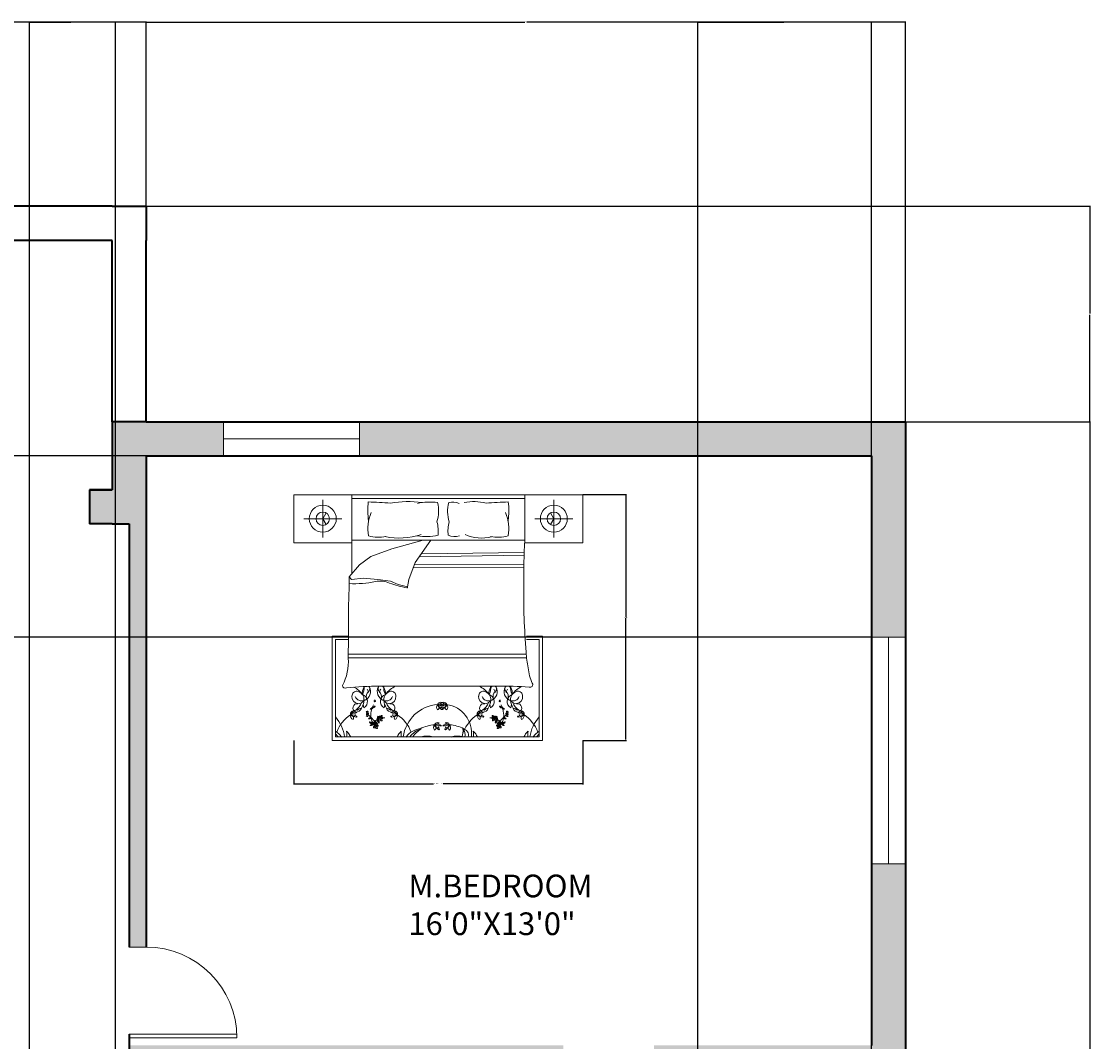
# Model space of a CAD drawing. Units: inches. Extents: x -26 to 13070, y -956 to 6917.
# Tile 11 of 13: x 314 to 597, y -154 to 116. Entities that reach past the tile are written whole.
import ezdxf

# ---------------------------------------------------------------- set-up
doc = ezdxf.new("R2010")
doc.units = ezdxf.units.IN
doc.header["$MEASUREMENT"] = 0
for name, color, linetype, lineweight in [('A-ANNO-DIMS', 2, 'Continuous', 18), ('A-AREA-IDEN', 7, 'Continuous', 18), ('A-DOOR', 3, 'Continuous', 18), ('A-FURN', 8, 'Continuous', 13), ('A-GLAZ', 4, 'Continuous', 18), ('A-WALL', 7, 'Continuous', 35), ('A-WALL-PATT', 252, 'Continuous', 13)]:
    doc.layers.add(name, color=color, linetype=linetype, lineweight=lineweight)
doc.styles.get("Standard").update_dxf_attribs({"font": 'arial.ttf'})
doc.dimstyles.get("Standard").update_dxf_attribs({"dimtxt": 0.18, "dimasz": 0.18, "dimexe": 0.18, "dimexo": 0.0625, "dimgap": 0.09, "dimtad": 0, "dimtih": 1, "dimtoh": 1, "dimdec": 0, "dimzin": 0, "dimdsep": 46, "dimlunit": 3, "dimtxsty": 'Standard', "dimcen": 0.09, "dimadec": 0, "dimazin": 0, "dimtfac": 1, "dimtdec": 0, "dimtofl": 0, "dimtmove": 0, "dimatfit": 3, "dimfxl": 1, "dimtolj": 1, "dimtzin": 0, "dimarcsym": 0})

# ---------------------------------------------------------------- blocks, each defined once
blk = doc.blocks.new('BED-DOUBLE-NIGHTSTANDS')
for p, q in [((0, 65), (76.43, 65)), ((7.64, 53.64), (7.64, 63.62)), ((15.29, 65), (15.29, 44.02)), ((61.14, 64.02), (15.29, 64.02)), ((68.79, 53.64), (68.79, 63.62)), ((12.64, 58.63), (2.65, 58.63)), ((63.79, 58.63), (73.78, 58.63)), ((15.29, 52.92), (61.14, 52.92)), ((25.9, 50.65), (34.24, 52.92)), ((36.28, 52.92), (32.09, 47.09)), ((17.39, 46.47), (20.33, 48.64)), ((20.33, 48.64), (25.9, 50.65)), ((60.91, 48.96), (33.16, 48.57)), ((60.94, 49.74), (33.73, 49.36)), ((14.6, 43.22), (17.39, 46.47)), ((32.09, 47.09), (30.39, 42.6)), ((60.87, 45.77), (31.55, 45.65)), ((60.87, 46.55), (31.85, 46.44)), ((15.22, 42.6), (14.6, 43.22)), ((18.32, 42.91), (15.22, 42.6)), ((22.19, 42.6), (18.32, 42.91)), ((25.59, 42.14), (22.19, 42.6)), ((30.39, 42.6), (30.08, 40.59)), ((27.6, 41.21), (25.59, 42.14)), ((30.08, 40.59), (27.6, 41.21)), ((10.09, 27.53), (14.41, 27.53)), ((10.09, 0), (10.09, 27.53)), ((14.41, 26.65), (10.97, 26.65)), ((10.97, 26.65), (10.97, 0.89)), ((64.92, 26.65), (61.55, 26.65)), ((61.57, 27.53), (65.81, 27.53)), ((64.92, 0.89), (64.92, 26.65)), ((65.81, 27.53), (65.81, 0)), ((61.49, 22.77), (14.41, 22.77)), ((61.56, 21.81), (14.4, 21.81)), ((53.73, 14.3), (22.7, 14.3)), ((18.51, 8.63), (18.34, 9.5)), ((23.85, 8.63), (24.02, 9.5)), ((52.05, 8.63), (51.88, 9.5)), ((57.39, 8.63), (57.56, 9.5)), ((10.97, 0.89), (64.92, 0.89)), ((65.81, 0), (10.09, 0))]:
    blk.add_line(p, q)
for points in [[(15.29, 52.26), (0, 52.26), (0, 65)], [(61.14, 65), (61.14, 52.26), (76.43, 52.26), (76.43, 65)], [(7.64, 58.63), (8.53, 60.17)], [(68.79, 58.63), (67.89, 60.17)], [(7.64, 58.63), (8.53, 57.08)], [(68.79, 58.63), (67.89, 57.08)]]:
    blk.add_lwpolyline(points)
for points in [[(19.68, 63.09, 0.074897), (19.77, 58.1, -0.472817)], [(37.86, 57.82, 0.14099), (38.01, 62.91, 0.235245)], [(41.12, 57.82, -0.14099), (40.97, 62.91, -0.235245)], [(56.75, 63.09, -0.074897), (56.66, 58.1, 0.472817)], [(14.44, 36.22, 0.001242), (14.4, 21.72, -0.127202), (12.87, 14.5)], [(61.47, 23.37, 0.056112), (62.02, 19.16, 0.095341), (63.1, 15.11)]]:
    blk.add_lwpolyline(points, format="xyb")
for centre, radius in [((7.64, 58.63), 3.57), ((7.64, 58.63), 1.78), ((68.79, 58.63), 3.57), ((68.79, 58.63), 1.78), ((22.92, 5.86), 0.195), ((52.98, 5.86), 0.195), ((21.65, 3.81), 0.195), ((54.25, 3.81), 0.195)]:
    blk.add_circle(centre, radius)
for centre, radius, start, end in [((61.8, 790.45), 728.57, 266.68521, 267.14978), ((30.15, 35.44), 27.72, 82.2196, 99.497), ((36, 49.44), 13.62, 81.5249, 103.96), ((42.02, 59.28), 3.78, 63.3437, 106.1026), ((47.68, 49.72), 13.44, 76.3427, 101.1841), ((14.63, 790.45), 728.57, 272.85022, 273.31479), ((29.41, 56.1), 9.85, 155.1316, 191.7583), ((47.02, 56.1), 9.85, 348.2417, 24.8684), ((28.85, 55.27), 9.36, 354.0129, 15.8293), ((50.13, 55.27), 9.36, 164.1707, 185.9871), ((22.4, 63.99), 10.24, 255.1039, 281.0369), ((27.79, 71.27), 17.76, 258.0397, 289.2615), ((34.99, 67.39), 13.48, 259.8617, 283.6238), ((42.53, 57.96), 4.05, 245.0183, 288.5407), ((49.61, 63.23), 9.73, 243.8761, 286.1746), ((54.03, 63.99), 10.24, 258.9631, 284.8961), ((198.16, 43.58), 137.33, 176.1, 180.9282), ((-55.48, 41.32), 70.1, 355.8294, 1.553), ((15.91, 70.29), 28.85, 267.4519, 281.3392), ((22.8, 35.91), 6.22, 66.2616, 101.3392), ((35.39, 69.47), 29.64, 250.1194, 259.3383), ((29.91, 40.53), 0.184, 268.8623, 19.7536), ((239.96, 38.59), 179.14, 179.1145, 184.8735), ((13.58, 14.54), 0.705, 183.98, 297.3412), ((21.79, -65.25), 79.56, 89.3433, 95.6887), ((15.4, 13.74), 3.17, 328.8218, 9.1554), ((19.32, 13.46), 0.92, 120.0293, 142.325), ((19.32, 13.46), 0.92, 44.4517, 63.558), ((23.03, 13.46), 0.92, 113.229, 135.5483), ((23.03, 13.46), 0.92, 37.675, 66.7144), ((26.95, 13.74), 3.17, 169.7133, 211.1782), ((29.07, 8.92), 5.78, 111.4941, 146.3329), ((46.82, 8.92), 5.78, 33.6671, 68.5059), ((48.94, 13.74), 3.17, 328.8218, 10.2867), ((52.87, 13.46), 0.92, 113.2856, 142.325), ((52.87, 13.46), 0.92, 44.4517, 66.7144), ((56.07, -60.03), 74.37, 85.2402, 91.8035), ((56.57, 13.46), 0.92, 106.6343, 135.5483), ((56.57, 13.46), 0.92, 37.675, 72.5814), ((60.5, 13.74), 3.17, 169.249, 211.1782), ((62.62, 8.92), 5.78, 113.6453, 146.3329), ((62.52, 14.72), 0.697, 246.5219, 33.8264), ((17.18, 11.52), 1.83, 174.9449, 262.8857), ((16.65, 11.7), 1.29, 84.4856, 181.0538), ((13.28, 8.92), 5.78, 33.6671, 63.2997), ((17.9, 12.21), 1.77, 201.5819, 291.4221), ((16.25, 10.75), 2.3, 355.2933, 76.921), ((21.03, 12.36), 2.95, 145.785, 184.7304), ((17.56, 10.28), 1.9, 299.9085, 73.1337), ((17.85, 12.92), 2.44, 289.2822, 29.1751), ((20.73, 11.61), 1.57, 131.5653, 195.1471), ((17.48, 12.48), 2.2, 7.436, 29.9149), ((18.93, 13.64), 1.14, 311.5653, 23.8354), ((24.5, 12.92), 2.44, 150.8249, 250.7178), ((23.42, 13.64), 1.14, 156.1646, 228.4347), ((21.62, 11.61), 1.57, 344.8529, 48.4347), ((24.87, 12.48), 2.2, 150.0851, 172.564), ((24.79, 10.28), 1.9, 106.8663, 240.0915), ((21.32, 12.36), 2.95, 355.2696, 34.215), ((26.1, 10.75), 2.3, 103.079, 184.7067), ((24.46, 12.21), 1.77, 248.5779, 338.4181), ((25.17, 11.52), 1.83, 277.1143, 5.0551), ((25.7, 11.7), 1.29, 358.9462, 95.5144), ((50.72, 11.52), 1.83, 174.9449, 262.8857), ((50.19, 11.7), 1.29, 84.4856, 181.0538), ((51.44, 12.21), 1.77, 201.5819, 291.4221), ((49.8, 10.75), 2.3, 355.2933, 76.921), ((54.57, 12.36), 2.95, 145.785, 184.7304), ((51.1, 10.28), 1.9, 299.9085, 73.1337), ((51.4, 12.92), 2.44, 289.2822, 29.1751), ((54.28, 11.61), 1.57, 131.5653, 195.1471), ((51.03, 12.48), 2.2, 7.436, 29.9149), ((52.48, 13.64), 1.14, 311.5653, 23.8354), ((58.04, 12.92), 2.44, 150.8249, 250.7178), ((56.96, 13.64), 1.14, 156.1646, 228.4347), ((55.16, 11.61), 1.57, 344.8529, 48.4347), ((58.41, 12.48), 2.2, 150.0851, 172.564), ((58.34, 10.28), 1.9, 106.8663, 240.0915), ((54.87, 12.36), 2.95, 355.2696, 34.215), ((59.64, 10.75), 2.3, 103.079, 184.7067), ((58, 12.21), 1.77, 248.5779, 338.4181), ((58.72, 11.52), 1.83, 277.1143, 5.0551), ((59.25, 11.7), 1.29, 358.9462, 95.5144), ((16.76, 8.57), 1.15, 80.264, 250.8688), ((14.48, 11.1), 3.61, 301.2614, 341.7045), ((16.48, 8.92), 1.43, 265.969, 344.3045), ((18.02, 7.01), 1.53, 96.1662, 141.5825), ((16.86, 11.92), 2.22, 272.3591, 324.0401), ((14.45, 10.81), 4.1, 326.2883, 356.5076), ((21.03, 12.36), 2.95, 212.7011, 216.3445), ((18.76, 11.08), 0.474, 257.3041, 15.1471), ((19.71, 9.44), 1.23, 308.2101, 316.3071), ((20.47, 8.64), 0.367, 278.3432, 4.2869), ((20.26, 8.96), 0.641, 300.656, 332.6341), ((20.74, 8.53), 0.156, 55.7657, 157.4417), ((26.69, 6.51), 6.33, 153.0032, 159.8941), ((20.99, 8.68), 0.156, 84.3784, 186.0543), ((20.84, 9.3), 0.641, 269.1859, 301.164), ((21.03, 8.97), 0.367, 237.5332, 323.4768), ((20.67, 10.02), 1.23, 285.5129, 293.6099), ((20.55, 9.79), 1.21, 301.164, 321.5612), ((21.48, 8.64), 0.401, 87.3579, 140.4944), ((21.4, 10.36), 0.147, 102.7051, 280.4384), ((19.56, 10), 2.16, 324.6898, 333.4936), ((21.38, 10.45), 0.24, 280.4384, 100.4136), ((23.59, 11.08), 0.474, 164.8529, 282.6959), ((21.32, 12.36), 2.95, 323.6555, 327.2989), ((25.49, 11.92), 2.22, 215.9599, 267.6409), ((27.9, 10.81), 4.1, 183.4924, 213.7117), ((27.87, 11.1), 3.61, 198.2955, 238.7386), ((24.33, 7.01), 1.53, 38.4175, 83.8338), ((25.87, 8.92), 1.43, 195.6955, 274.031), ((25.59, 8.57), 1.15, 289.1312, 99.736), ((38.81, -0.46), 9.98, 94.4623, 172.255), ((38.85, 8.75), 1.11, 137.7873, 219.1145), ((37.6, 8.78), 0.834, 298.5391, 58.3627), ((38.83, 9.26), 0.827, 63.0274, 163.8037), ((37.99, 11.2), 1.7, 271.4585, 315.3727), ((38.68, 8.05), 1.58, 45.5411, 114.3101), ((40.12, 16.15), 6.98, 252.593, 267.2582), ((38.85, 9.46), 0.816, 177.7585, 283.852), ((40.42, 10.31), 2.52, 198.9159, 238.011), ((39.76, 8.05), 1.58, 65.6899, 134.4589), ((38.32, 16.15), 6.98, 272.7418, 287.407), ((39.02, 8.77), 0.108, 283.852, 219.9245), ((39.62, 9.26), 0.827, 16.1963, 116.9726), ((40.45, 11.2), 1.7, 224.6273, 268.5415), ((39.42, 8.81), 0.0651, 320.1909, 256.0209), ((38.02, 10.31), 2.52, 301.989, 341.0841), ((39.6, 9.46), 0.816, 256.148, 2.2415), ((40.85, 8.78), 0.834, 121.6373, 241.4609), ((39.59, 8.75), 1.11, 320.8855, 42.2127), ((39.31, 1.85), 7.72, 352.8636, 81.8197), ((50.3, 8.57), 1.15, 80.264, 250.8688), ((48.03, 11.1), 3.61, 301.2614, 341.7045), ((50.03, 8.92), 1.43, 265.969, 344.3045), ((51.57, 7.01), 1.53, 96.1662, 141.5825), ((50.4, 11.92), 2.22, 272.3591, 324.0401), ((47.99, 10.81), 4.1, 326.2883, 356.5076), ((54.57, 12.36), 2.95, 212.7011, 216.3445), ((52.3, 11.08), 0.474, 257.3041, 15.1471), ((54.52, 10.45), 0.24, 79.5864, 259.5616), ((55.35, 9.79), 1.21, 218.4388, 238.836), ((54.42, 8.64), 0.401, 39.5056, 92.6421), ((56.33, 10), 2.16, 206.5064, 215.3102), ((54.5, 10.36), 0.147, 259.5616, 77.2949), ((54.87, 8.97), 0.367, 216.5232, 302.4668), ((55.05, 9.3), 0.641, 238.836, 270.8141), ((55.22, 10.02), 1.23, 246.3901, 254.4871), ((49.2, 6.51), 6.33, 20.1059, 26.9968), ((54.91, 8.68), 0.156, 353.9457, 95.6216), ((55.15, 8.53), 0.156, 22.5583, 124.2343), ((55.43, 8.64), 0.367, 175.7131, 261.6568), ((55.63, 8.96), 0.641, 207.3659, 239.344), ((56.18, 9.44), 1.23, 223.6929, 231.7899), ((57.13, 11.08), 0.474, 164.8529, 282.6959), ((54.87, 12.36), 2.95, 323.6555, 327.2989), ((59.04, 11.92), 2.22, 215.9599, 267.6409), ((61.45, 10.81), 4.1, 183.4924, 213.7117), ((61.41, 11.1), 3.61, 198.2955, 238.7386), ((59.41, 8.92), 1.43, 195.6955, 274.031), ((57.87, 7.01), 1.53, 38.4175, 83.8338), ((59.14, 8.57), 1.15, 289.1312, 99.736), ((3.54, -0.46), 9.98, 7.745, 41.8856), ((20.62, -1.45), 9.98, 124.3865, 158.5908), ((15.79, 6.99), 0.827, 92.9516, 193.728), ((16.06, 6.55), 1.11, 167.7115, 249.0387), ((14.09, 8.25), 1.7, 301.3827, 345.2969), ((16.26, 5.87), 1.58, 75.4653, 144.2343), ((13.47, 13.61), 6.98, 282.5173, 297.1824), ((14.96, 5.96), 0.834, 328.4633, 88.2869), ((16.64, 8.69), 2.52, 228.8402, 267.9352), ((15.7, 7.17), 0.816, 207.6827, 313.7762), ((16.52, 7.33), 0.703, 63.9755, 143.2681), ((16.19, 6.66), 0.108, 313.7762, 249.7183), ((16.54, 6.35), 0.0602, 101.4834, 217.9409), ((16.56, 6.29), 0.124, 267.9352, 101.4834), ((19.42, 7.32), 0.325, 101.5637, 142.6358), ((19.15, 7.02), 0.195, 273.2768, 86.7232), ((19.41, 6.66), 0.321, 217.7621, 259.0403), ((19.37, 7.21), 0.186, 91.1081, 181.8675), ((19.76, 7.09), 0.591, 203.4276, 227.6104), ((19.57, 6.83), 0.402, 80.3487, 133.6538), ((19.5, 7.16), 0.318, 229.7889, 317.6792), ((19.16, 7.58), 0.468, 288.7263, 352.5032), ((19.14, 6.49), 0.452, 355.053, 68.3618), ((19.5, 6.41), 0.637, 83.0852, 105.7171), ((19.47, 7.55), 0.15, 345.2356, 144.9248), ((19.44, 6.46), 0.149, 232.4737, 355.053), ((15.08, 1.13), 7.26, 43.1541, 52.0459), ((19.61, 7.06), 0.168, 317.6792, 80.3487), ((20.1, 5.51), 0.401, 101.3256, 154.4621), ((19.52, 6.87), 1.21, 280.2588, 300.656), ((19.8, 7.84), 2.16, 268.3264, 277.1302), ((19.26, 6.87), 1.23, 308.2101, 316.3071), ((20.01, 6.06), 0.367, 278.3432, 4.2869), ((19.81, 6.39), 0.641, 300.656, 332.6341), ((20.29, 5.96), 0.156, 55.7657, 157.4417), ((20.55, 8.08), 0.401, 101.3256, 154.4621), ((19.97, 9.45), 1.21, 280.2588, 300.656), ((20.25, 10.41), 2.16, 268.3264, 277.1302), ((26.69, 6.51), 6.33, 163.5842, 183.8277), ((23.54, 6.35), 3.17, 184.756, 209.2041), ((28.11, 13.11), 10.44, 222.2412, 232.1744), ((21.43, 6.15), 0.887, 304.5369, 16.3699), ((21.9, 5.96), 0.539, 272.8499, 356.1226), ((21.52, 5.75), 0.522, 321.7607, 7.9252), ((22.66, 5.9), 0.628, 127.3105, 187.9252), ((21.8, 5.98), 0.645, 355.0106, 41.658), ((22.87, 5.28), 0.614, 104.7558, 148.0499), ((22.71, 6.14), 0.265, 126.1046, 271.4281), ((22.68, 6.21), 0.191, 353.7526, 131.7054), ((22.63, 5.7), 0.129, 262.906, 7.132), ((22.5, 5.98), 0.268, 0.0645, 61.1507), ((22.56, 6.21), 0.306, 311.8413, 355.7877), ((23.19, 6.17), 0.325, 101.5637, 176.365), ((23.15, 6.05), 0.186, 91.1081, 181.8675), ((23.53, 5.93), 0.591, 203.4276, 227.6104), ((23.35, 5.67), 0.402, 80.3487, 133.6538), ((23.27, 6.01), 0.318, 229.7889, 317.6792), ((22.93, 6.42), 0.468, 288.7263, 352.5032), ((22.91, 5.33), 0.452, 355.053, 68.3618), ((23.27, 5.26), 0.637, 83.0852, 105.7171), ((23.25, 6.4), 0.15, 345.2356, 144.9248), ((23.38, 5.91), 0.168, 317.6792, 80.3487), ((23.87, 2.14), 3.81, 87.1071, 94.7585), ((25.83, 7.33), 0.703, 36.7319, 116.0245), ((25.8, 6.29), 0.124, 78.5166, 272.0648), ((26.09, 5.87), 1.58, 35.7657, 104.5347), ((28.88, 13.61), 6.98, 242.8176, 257.4827), ((25.71, 8.69), 2.52, 272.0648, 311.1598), ((25.81, 6.35), 0.0602, 322.0591, 78.5166), ((26.65, 7.17), 0.816, 226.2238, 332.3173), ((26.17, 6.7), 0.0651, 290.2667, 226.2271), ((27.4, 5.96), 0.834, 91.7131, 211.5367), ((26.57, 6.99), 0.827, 346.272, 87.0484), ((28.26, 8.25), 1.7, 194.7031, 238.6173), ((26.29, 6.55), 1.11, 290.9613, 12.2885), ((21.73, -1.45), 9.98, 21.4092, 55.6135), ((39.15, 8.27), 0.124, 238.011, 71.5592), ((39.17, 8.33), 0.0602, 71.5592, 188.0167), ((39.29, 8.27), 0.124, 108.4408, 301.989), ((39.27, 8.33), 0.0602, 351.9833, 108.4408), ((54.16, -1.45), 9.98, 124.3865, 158.5908), ((49.33, 6.99), 0.827, 92.9516, 193.728), ((49.61, 6.55), 1.11, 167.7115, 249.0387), ((47.64, 8.25), 1.7, 301.3827, 345.2969), ((49.81, 5.87), 1.58, 75.4653, 144.2343), ((47.01, 13.61), 6.98, 282.5173, 297.1824), ((49.25, 7.17), 0.816, 207.6827, 313.7762), ((50.19, 8.69), 2.52, 228.8402, 267.9352), ((48.5, 5.96), 0.834, 328.4633, 88.2869), ((50.06, 7.33), 0.703, 63.9755, 143.2681), ((49.74, 6.66), 0.108, 313.7762, 249.7183), ((50.09, 6.35), 0.0602, 101.4834, 217.9409), ((50.1, 6.29), 0.124, 267.9352, 101.4834), ((52.03, 2.14), 3.81, 85.2415, 92.8929), ((52.51, 5.91), 0.168, 99.6513, 222.3208), ((52.62, 6.01), 0.318, 222.3208, 310.2111), ((52.55, 5.67), 0.402, 46.3462, 99.6513), ((52.65, 6.4), 0.15, 35.0752, 194.7644), ((52.97, 6.42), 0.468, 187.4968, 251.2737), ((52.98, 5.33), 0.452, 111.6382, 184.947), ((52.63, 5.26), 0.637, 74.2829, 96.9148), ((52.75, 6.05), 0.186, 358.1325, 88.8919), ((52.36, 5.93), 0.591, 312.3896, 336.5724), ((52.71, 6.17), 0.325, 3.635, 78.4363), ((53.22, 6.21), 0.191, 48.2946, 186.2474), ((53.34, 6.21), 0.306, 184.2123, 228.1587), ((53.4, 5.98), 0.268, 118.8493, 179.9355), ((53.26, 5.7), 0.129, 172.868, 277.094), ((53.19, 6.14), 0.265, 268.5719, 53.8954), ((53.03, 5.28), 0.614, 31.9501, 75.2442), ((54.1, 5.98), 0.645, 138.342, 184.9894), ((53.99, 5.96), 0.539, 183.8774, 267.1501), ((54.47, 6.15), 0.887, 163.6301, 235.4631), ((53.23, 5.9), 0.628, 352.0748, 52.6895), ((54.37, 5.75), 0.522, 172.0748, 218.2393), ((47.79, 13.11), 10.44, 307.8256, 317.7588), ((52.36, 6.35), 3.17, 330.7959, 355.244), ((49.2, 6.51), 6.33, 356.1723, 16.4158), ((55.92, 9.45), 1.21, 239.344, 259.7412), ((55.64, 10.41), 2.16, 262.8698, 271.6736), ((55.34, 8.08), 0.401, 25.5379, 78.6744), ((60.81, 1.13), 7.26, 127.9541, 136.8459), ((55.61, 5.96), 0.156, 22.5583, 124.2343), ((55.88, 6.06), 0.367, 175.7131, 261.6568), ((56.09, 6.39), 0.641, 207.3659, 239.344), ((56.64, 6.87), 1.23, 223.6929, 231.7899), ((56.38, 6.87), 1.21, 239.344, 259.7412), ((56.1, 7.84), 2.16, 262.8698, 271.6736), ((55.8, 5.51), 0.401, 25.5379, 78.6744), ((56.28, 7.06), 0.168, 99.6513, 222.3208), ((56.4, 7.16), 0.318, 222.3208, 310.2111), ((56.32, 6.83), 0.402, 46.3462, 99.6513), ((56.42, 7.55), 0.15, 35.0752, 194.7644), ((56.74, 7.58), 0.468, 187.4968, 251.2737), ((56.76, 6.49), 0.452, 111.6382, 184.947), ((56.45, 6.46), 0.149, 184.947, 307.5263), ((56.4, 6.41), 0.637, 74.2829, 96.9148), ((56.52, 7.21), 0.186, 358.1325, 88.8919), ((56.14, 7.09), 0.591, 312.3896, 336.5724), ((56.48, 7.32), 0.325, 37.3642, 78.4363), ((56.48, 6.66), 0.321, 280.9597, 322.2379), ((56.75, 7.02), 0.195, 93.2768, 266.7232), ((59.37, 7.33), 0.703, 36.7319, 116.0245), ((59.34, 6.29), 0.124, 78.5166, 272.0648), ((59.63, 5.87), 1.58, 35.7657, 104.5347), ((62.43, 13.61), 6.98, 242.8176, 257.4827), ((59.25, 8.69), 2.52, 272.0648, 311.1598), ((59.35, 6.35), 0.0602, 322.0591, 78.5166), ((60.19, 7.17), 0.816, 226.2238, 332.3173), ((59.71, 6.7), 0.0651, 290.2667, 226.2271), ((60.94, 5.96), 0.834, 91.7131, 211.5367), ((61.8, 8.25), 1.7, 194.7031, 238.6173), ((60.11, 6.99), 0.827, 346.272, 87.0484), ((59.83, 6.55), 1.11, 290.9613, 12.2885), ((55.28, -1.45), 9.98, 21.4092, 55.6135), ((72.35, -0.46), 9.98, 138.1144, 172.255), ((20.23, 4.81), 0.217, 146.8636, 236.9021), ((23.3, 9.6), 5.69, 235.1882, 238.8844), ((20.6, 5.12), 0.588, 199.4799, 267.6828), ((20.54, 4.9), 0.507, 212.8155, 277.3992), ((20.24, 4.56), 0.588, 266.9701, 338.2913), ((17.14, 8.76), 5.69, 302.6784, 306.3746), ((20.39, 4.1), 0.217, 214.3538, 304.3923), ((20.47, 4.92), 0.225, 238.8844, 314.2646), ((20.42, 4.42), 0.507, 280.3057, 17.1958), ((20.38, 4.36), 0.225, 306.3746, 21.7548), ((20.75, 4.51), 0.17, 19.3605, 201.7548), ((20.75, 4.64), 0.17, 311.8703, 134.2646), ((23.94, 3.09), 3.39, 153.7819, 158.2913), ((21.24, 5.41), 0.887, 247.2305, 319.0635), ((20.95, 5.11), 0.522, 264.4544, 310.6188), ((23.54, 6.35), 3.17, 214.0033, 222.4917), ((21.33, 4.9), 0.539, 218.3208, 298.8162), ((23.87, 2.14), 3.81, 120.544, 139.818), ((21.24, 3.45), 0.193, 148.0499, 225.6268), ((21.6, 3.23), 0.614, 104.7558, 148.0499), ((21.25, 3.66), 0.384, 247.4086, 351.4386), ((21.43, 4.08), 0.265, 126.1046, 271.4281), ((21.4, 4.16), 0.191, 353.7526, 131.7054), ((21.7, 4.23), 0.628, 70.0041, 130.6188), ((21.36, 3.65), 0.129, 262.906, 7.132), ((21.22, 3.93), 0.268, 0.0645, 61.1507), ((21.29, 4.16), 0.306, 311.8413, 355.7877), ((21.29, 5), 0.645, 297.7043, 344.3516), ((21.92, 4.11), 0.325, 101.5637, 176.365), ((21.91, 3.45), 0.321, 151.2196, 259.0403), ((21.87, 4), 0.186, 91.1081, 181.8675), ((22.26, 3.88), 0.591, 203.4276, 227.6104), ((22.07, 3.62), 0.402, 80.3487, 133.6538), ((22, 3.96), 0.318, 229.7889, 317.6792), ((21.66, 4.37), 0.468, 288.7263, 352.5032), ((21.64, 3.28), 0.452, 355.053, 68.3618), ((22, 3.21), 0.637, 83.0852, 105.7171), ((21.97, 4.35), 0.15, 345.2356, 144.9248), ((21.94, 3.26), 0.149, 232.4737, 355.053), ((21.63, 5), 0.522, 8.7227, 54.8872), ((21.66, 4.58), 0.887, 0.278, 72.111), ((22.06, 4.9), 0.539, 20.5253, 88.5375), ((22.11, 3.85), 0.168, 317.6792, 80.3487), ((22.77, 5.17), 0.628, 188.7227, 249.3375), ((22.51, 5.5), 0.193, 148.0499, 225.6268), ((23.87, 2.14), 3.81, 113.0501, 113.8477), ((22.52, 5.72), 0.384, 247.4086, 351.4386), ((21.96, 4.86), 0.645, 334.9899, 21.6373), ((23.19, 5.5), 0.321, 151.2196, 259.0403), ((23.22, 5.31), 0.149, 232.4737, 355.053), ((33.8, -1.8), 4.86, 91.272, 146.5383), ((35.55, -2.7), 6.06, 107.8504, 143.6964), ((38.74, -4.41), 9.02, 124.0123, 144.053), ((38.04, -5.81), 9.98, 94.4623, 117.4146), ((38.09, 3.4), 1.11, 137.7873, 219.1145), ((36.83, 3.44), 0.834, 298.5391, 58.3627), ((38.06, 3.91), 0.827, 63.0274, 163.8037), ((37.22, 5.85), 1.7, 271.4585, 315.3727), ((37.92, 2.71), 1.58, 45.5411, 114.3101), ((39.66, 4.96), 2.52, 198.9159, 238.011), ((39.36, 10.81), 6.98, 252.593, 267.2582), ((38.08, 4.11), 0.816, 177.7585, 283.852), ((38.25, 3.43), 0.108, 283.852, 219.9245), ((38.38, 2.93), 0.124, 238.011, 71.5592), ((38.4, 2.99), 0.0602, 71.5592, 188.0167), ((40.53, 2.71), 1.58, 65.6899, 134.4589), ((39.09, 10.81), 6.98, 272.7418, 287.407), ((40.06, 2.93), 0.124, 108.4408, 301.989), ((40.38, 3.91), 0.827, 16.1963, 116.9726), ((41.22, 5.85), 1.7, 224.6273, 268.5415), ((40.04, 2.99), 0.0602, 351.9833, 108.4408), ((40.18, 3.47), 0.0651, 320.1909, 256.0209), ((38.79, 4.96), 2.52, 301.989, 341.0841), ((40.36, 4.11), 0.816, 256.148, 2.2415), ((41.61, 3.44), 0.834, 121.6373, 241.4609), ((40.36, 3.4), 1.11, 320.8855, 42.2127), ((40.4, -5.81), 9.98, 62.5854, 85.5377), ((40.31, 2.55), 4.47, 338.117, 6.6195), ((44.41, 1.31), 1.79, 346.3898, 79.0739), ((43.06, 1.55), 2.27, 342.8609, 41.9049), ((52.68, 5.31), 0.149, 184.947, 307.5263), ((52.71, 5.5), 0.321, 280.9597, 28.7804), ((53.37, 5.72), 0.384, 188.5614, 292.5914), ((53.93, 4.86), 0.645, 158.3627, 205.0101), ((53.84, 4.9), 0.539, 91.4625, 159.4747), ((54.23, 4.58), 0.887, 107.889, 179.722), ((53.13, 5.17), 0.628, 290.6625, 351.2773), ((52.03, 2.14), 3.81, 66.1523, 66.9499), ((53.38, 5.5), 0.193, 314.3732, 31.9501), ((53.78, 3.85), 0.168, 99.6513, 222.3208), ((53.9, 3.96), 0.318, 222.3208, 310.2111), ((54.26, 5), 0.522, 125.1128, 171.2773), ((53.82, 3.62), 0.402, 46.3462, 99.6513), ((53.92, 4.35), 0.15, 35.0752, 194.7644), ((54.24, 4.37), 0.468, 187.4968, 251.2737), ((54.26, 3.28), 0.452, 111.6382, 184.947), ((53.95, 3.26), 0.149, 184.947, 307.5263), ((53.9, 3.21), 0.637, 74.2829, 96.9148), ((52.03, 2.14), 3.81, 40.182, 59.456), ((54.2, 4.23), 0.628, 49.3812, 109.9959), ((54.65, 5.41), 0.887, 220.9365, 292.7695), ((54.6, 5), 0.645, 195.6484, 242.2957), ((54.02, 4), 0.186, 358.1325, 88.8919), ((53.64, 3.88), 0.591, 312.3896, 336.5724), ((53.98, 4.11), 0.325, 3.635, 78.4363), ((53.98, 3.45), 0.321, 280.9597, 28.7804), ((54.64, 3.66), 0.384, 188.5614, 292.5914), ((54.56, 4.9), 0.539, 241.1838, 321.6792), ((54.49, 4.16), 0.191, 48.2946, 186.2474), ((54.61, 4.16), 0.306, 184.2123, 228.1587), ((54.67, 3.93), 0.268, 118.8493, 179.9355), ((54.54, 3.65), 0.129, 172.868, 277.094), ((54.46, 4.08), 0.265, 268.5719, 53.8954), ((54.3, 3.23), 0.614, 31.9501, 75.2442), ((54.95, 5.11), 0.522, 229.3812, 275.5456), ((52.36, 6.35), 3.17, 317.5083, 325.9967), ((54.66, 3.45), 0.193, 314.3732, 31.9501), ((55.47, 4.42), 0.507, 162.8042, 259.6943), ((55.15, 4.64), 0.17, 45.7354, 228.1297), ((55.15, 4.51), 0.17, 338.2452, 160.6395), ((51.96, 3.09), 3.39, 21.7087, 26.2181), ((55.65, 4.56), 0.588, 201.7087, 273.0299), ((55.42, 4.92), 0.225, 225.7354, 301.1156), ((55.36, 4.9), 0.507, 262.6008, 327.1845), ((55.51, 4.36), 0.225, 158.2452, 233.6254), ((55.29, 5.12), 0.588, 272.3172, 340.5201), ((58.75, 8.76), 5.69, 233.6254, 237.3216), ((55.5, 4.1), 0.217, 235.6077, 325.6462), ((52.6, 9.6), 5.69, 301.1156, 304.8118), ((55.66, 4.81), 0.217, 303.0979, 33.1364), ((8.55, -1.8), 4.86, 33.4617, 60.1116), ((6.8, -2.7), 6.06, 36.3036, 46.4814), ((11.27, -0.67), 4.06, 22.5547, 48.9546), ((0.16, 1.51), 13.81, 357.4081, 3.6519), ((31.08, -0.67), 4.06, 131.0454, 157.4453), ((42.19, 1.51), 13.81, 176.3481, 182.5919), ((35.25, -4.36), 5.49, 73.5431, 107.0202), ((37.43, -7.19), 8.12, 94.3787, 95.6357), ((41.7, -12.75), 14.5, 109.7217, 109.9028), ((43.19, -4.36), 5.49, 72.9798, 106.4569), ((41.02, -7.19), 8.12, 84.3643, 85.6213), ((36.74, -12.75), 14.5, 70.0972, 70.2783), ((33.7, 1.51), 13.81, 357.4081, 3.6519), ((44.82, -0.67), 4.06, 22.5547, 48.9546), ((64.62, -0.67), 4.06, 131.0454, 157.4453), ((75.74, 1.51), 13.81, 176.3481, 182.5919), ((67.35, -1.8), 4.86, 119.8884, 146.5383), ((69.1, -2.7), 6.06, 133.5186, 143.6964)]:
    blk.add_arc(centre, radius, start, end)
blk = doc.blocks.new('DOOR-SWING-24')
for p, q in [((24, 1), (0, 1)), ((24, 0), (0, 0))]:
    blk.add_line(p, q)
blk.add_arc((24, 0), 24, 90, 180)
blk = doc.blocks.new('WIN-36')
for p, q in [((0, 36), (0, 0)), ((9, 36), (0, 36)), ((4.5, 36), (4.5, 0)), ((9, 0), (9, 36)), ((0, 0), (9, 0))]:
    blk.add_line(p, q)
blk = doc.blocks.new('WIN-60')
for p, q in [((0, 0), (0, 60)), ((0, 60), (9, 60)), ((4.5, 0), (4.5, 60)), ((9, 60), (9, 0)), ((9, 0), (0, 0))]:
    blk.add_line(p, q)
blk = doc.blocks.new('*D26')
at = {"layer": 'A-ANNO-DIMS', "color": 0, "lineweight": -2, "transparency": 16777216}
for p, q in [((385.73, -73.89), (385.73, -85.48)), ((462.16, -73.89), (462.16, -85.48)), ((385.91, -85.3), (422.63, -85.3)), ((461.98, -85.3), (425.26, -85.3))]:
    blk.add_line(p, q, dxfattribs=at)
at = {"layer": 'A-ANNO-DIMS', "color": 0, "transparency": 16777216}
for points in [[(385.91, -85.27), (385.91, -85.33), (385.73, -85.3)], [(461.98, -85.27), (461.98, -85.33), (462.16, -85.3)]]:
    blk.add_solid(points, dxfattribs=at)
at = {"layer": 'Defpoints', "color": 0, "transparency": 16777216}
for p in [(385.73, -73.83), (462.16, -73.83), (462.16, -85.3)]:
    blk.add_point(p, dxfattribs=at)
at = {"layer": 'A-ANNO-DIMS', "color": 0, "transparency": 16777216, "insert": (423.94, -85.3), "char_height": 0.18, "attachment_point": 5}
blk.add_mtext('\\A1;BED GROUP 76 TYP.', dxfattribs=at)
blk = doc.blocks.new('*D27')
at = {"layer": 'A-ANNO-DIMS', "color": 0, "lineweight": -2, "transparency": 16777216}
for p, q in [((462.22, -8.83), (473.8, -8.83)), ((473.62, -9.01), (473.62, -41.15)), ((473.62, -73.65), (473.62, -41.52)), ((462.22, -73.83), (473.8, -73.83))]:
    blk.add_line(p, q, dxfattribs=at)
at = {"layer": 'A-ANNO-DIMS', "color": 0, "transparency": 16777216}
for points in [[(473.59, -9.01), (473.65, -9.01), (473.62, -8.83)], [(473.59, -73.65), (473.65, -73.65), (473.62, -73.83)]]:
    blk.add_solid(points, dxfattribs=at)
at = {"layer": 'Defpoints', "color": 0, "transparency": 16777216}
for p in [(462.16, -8.83), (473.62, -8.83), (462.16, -73.83)]:
    blk.add_point(p, dxfattribs=at)
at = {"layer": 'A-ANNO-DIMS', "color": 0, "transparency": 16777216, "insert": (473.62, -41.33), "char_height": 0.18, "attachment_point": 5}
blk.add_mtext('\\A1;65 TYP.', dxfattribs=at)
blk = doc.blocks.new('*D43')
at = {"layer": 'A-ANNO-DIMS', "color": 0, "lineweight": -2, "transparency": 16777216}
for p, q in [((214.64, 67.52), (214.64, 116.39)), ((214.82, 116.21), (280.36, 116.21)), ((346.46, 116.21), (280.92, 116.21)), ((346.64, 67.52), (346.64, 116.39))]:
    blk.add_line(p, q, dxfattribs=at)
at = {"layer": 'A-ANNO-DIMS', "color": 0, "transparency": 16777216}
for points in [[(214.82, 116.24), (214.82, 116.18), (214.64, 116.21)], [(346.46, 116.24), (346.46, 116.18), (346.64, 116.21)]]:
    blk.add_solid(points, dxfattribs=at)
at = {"layer": 'Defpoints', "color": 0, "transparency": 16777216}
for p in [(346.64, 116.21), (214.64, 67.46), (346.64, 67.46)]:
    blk.add_point(p, dxfattribs=at)
at = {"layer": 'A-ANNO-DIMS', "color": 0, "transparency": 16777216, "insert": (280.64, 116.21), "char_height": 0.18, "attachment_point": 5}
blk.add_mtext('\\A1;132', dxfattribs=at)
blk = doc.blocks.new('*D44')
at = {"layer": 'A-ANNO-DIMS', "color": 0, "lineweight": -2, "transparency": 16777216}
for p, q in [((346.64, 67.52), (346.64, 116.39)), ((346.82, 116.21), (446.87, 116.21)), ((547.46, 116.21), (447.41, 116.21)), ((547.64, 10.52), (547.64, 116.39))]:
    blk.add_line(p, q, dxfattribs=at)
at = {"layer": 'A-ANNO-DIMS', "color": 0, "transparency": 16777216}
for points in [[(346.82, 116.24), (346.82, 116.18), (346.64, 116.21)], [(547.46, 116.24), (547.46, 116.18), (547.64, 116.21)]]:
    blk.add_solid(points, dxfattribs=at)
at = {"layer": 'Defpoints', "color": 0, "transparency": 16777216}
for p in [(547.64, 116.21), (346.64, 67.46), (547.64, 10.46)]:
    blk.add_point(p, dxfattribs=at)
at = {"layer": 'A-ANNO-DIMS', "color": 0, "transparency": 16777216, "insert": (447.14, 116.21), "char_height": 0.18, "attachment_point": 5}
blk.add_mtext('\\A1;201', dxfattribs=at)
blk = doc.blocks.new('*D45')
at = {"layer": 'A-ANNO-DIMS', "color": 0, "lineweight": -2, "transparency": 16777216}
for p, q in [((547.7, 10.46), (596.57, 10.46)), ((596.39, 10.28), (596.39, -223.36)), ((596.39, -457.36), (596.39, -223.72)), ((538.7, -457.54), (596.57, -457.54))]:
    blk.add_line(p, q, dxfattribs=at)
at = {"layer": 'A-ANNO-DIMS', "color": 0, "transparency": 16777216}
for points in [[(596.36, 10.28), (596.42, 10.28), (596.39, 10.46)], [(596.36, -457.36), (596.42, -457.36), (596.39, -457.54)]]:
    blk.add_solid(points, dxfattribs=at)
at = {"layer": 'Defpoints', "color": 0, "transparency": 16777216}
for p in [(547.64, 10.46), (596.39, 10.46), (538.64, -457.54)]:
    blk.add_point(p, dxfattribs=at)
at = {"layer": 'A-ANNO-DIMS', "color": 0, "transparency": 16777216, "insert": (596.39, -223.54), "char_height": 0.18, "attachment_point": 5}
blk.add_mtext('\\A1;468', dxfattribs=at)
blk = doc.blocks.new('*D47')
at = {"layer": 'A-ANNO-DIMS', "color": 0, "lineweight": -2, "transparency": 16777216}
for p, q in [((346.7, 67.46), (596.57, 67.46)), ((596.39, 67.28), (596.39, 39.14)), ((596.39, 10.64), (596.39, 38.78)), ((547.7, 10.46), (596.57, 10.46))]:
    blk.add_line(p, q, dxfattribs=at)
at = {"layer": 'A-ANNO-DIMS', "color": 0, "transparency": 16777216}
for points in [[(596.36, 67.28), (596.42, 67.28), (596.39, 67.46)], [(596.36, 10.64), (596.42, 10.64), (596.39, 10.46)]]:
    blk.add_solid(points, dxfattribs=at)
at = {"layer": 'Defpoints', "color": 0, "transparency": 16777216}
for p in [(346.64, 67.46), (596.39, 67.46), (547.64, 10.46)]:
    blk.add_point(p, dxfattribs=at)
at = {"layer": 'A-ANNO-DIMS', "color": 0, "transparency": 16777216, "insert": (596.39, 38.96), "char_height": 0.18, "attachment_point": 5}
blk.add_mtext('\\A1;57', dxfattribs=at)
blk = doc.blocks.new('*D50')
at = {"layer": 'A-ANNO-DIMS', "color": 0, "lineweight": -2, "transparency": 16777216}
for p, q in [((315.7, -495.61), (315.7, 116.39)), ((315.88, 116.21), (326.72, 116.21)), ((338.35, 116.21), (327.51, 116.21)), ((338.53, -495.61), (338.53, 116.39))]:
    blk.add_line(p, q, dxfattribs=at)
at = {"layer": 'A-ANNO-DIMS', "color": 0, "transparency": 16777216}
for points in [[(315.88, 116.24), (315.88, 116.18), (315.7, 116.21)], [(338.35, 116.24), (338.35, 116.18), (338.53, 116.21)]]:
    blk.add_solid(points, dxfattribs=at)
at = {"layer": 'Defpoints', "color": 0, "transparency": 16777216}
for p in [(338.53, 116.21), (315.7, -495.67), (338.53, -495.67)]:
    blk.add_point(p, dxfattribs=at)
at = {"layer": 'A-ANNO-DIMS', "color": 0, "transparency": 16777216, "insert": (327.12, 116.21), "char_height": 0.18, "attachment_point": 5}
blk.add_mtext('\\A1;22.83', dxfattribs=at)
blk = doc.blocks.new('*D53')
at = {"layer": 'A-ANNO-DIMS', "color": 0, "lineweight": -2, "transparency": 16777216}
for p, q in [((492.64, -622.48), (492.64, 116.39)), ((492.82, 116.21), (515.42, 116.21)), ((538.46, 116.21), (515.86, 116.21)), ((538.64, -622.48), (538.64, 116.39))]:
    blk.add_line(p, q, dxfattribs=at)
at = {"layer": 'A-ANNO-DIMS', "color": 0, "transparency": 16777216}
for points in [[(492.82, 116.24), (492.82, 116.18), (492.64, 116.21)], [(538.46, 116.24), (538.46, 116.18), (538.64, 116.21)]]:
    blk.add_solid(points, dxfattribs=at)
at = {"layer": 'Defpoints', "color": 0, "transparency": 16777216}
for p in [(538.64, 116.21), (492.64, -622.54), (538.64, -622.54)]:
    blk.add_point(p, dxfattribs=at)
at = {"layer": 'A-ANNO-DIMS', "color": 0, "transparency": 16777216, "insert": (515.64, 116.21), "char_height": 0.18, "attachment_point": 5}
blk.add_mtext('\\A1;46', dxfattribs=at)
blk = doc.blocks.new('*D58')
at = {"layer": 'A-ANNO-DIMS', "color": 0, "lineweight": -2, "transparency": 16777216}
for p, q in [((538.58, 1.46), (-26.29, 1.46)), ((-26.11, 1.28), (-26.11, -22.36)), ((-26.11, -46.36), (-26.11, -22.72)), ((538.58, -46.54), (-26.29, -46.54))]:
    blk.add_line(p, q, dxfattribs=at)
at = {"layer": 'A-ANNO-DIMS', "color": 0, "transparency": 16777216}
for points in [[(-26.14, 1.28), (-26.08, 1.28), (-26.11, 1.46)], [(-26.14, -46.36), (-26.08, -46.36), (-26.11, -46.54)]]:
    blk.add_solid(points, dxfattribs=at)
at = {"layer": 'Defpoints', "color": 0, "transparency": 16777216}
for p in [(-26.11, 1.46), (538.64, 1.46), (538.64, -46.54)]:
    blk.add_point(p, dxfattribs=at)
at = {"layer": 'A-ANNO-DIMS', "color": 0, "transparency": 16777216, "insert": (-26.11, -22.54), "char_height": 0.18, "attachment_point": 5}
blk.add_mtext('\\A1;48', dxfattribs=at)

msp = doc.modelspace()

# ---------------------------------------------------------------- hatches: boundary and pattern name
at = {"layer": 'A-WALL-PATT'}
h = msp.add_hatch(color=256, dxfattribs=at)
h.dxf.hatch_style = 1
h.paths.add_polyline_path([(223.641, 10.458), (214.641, 10.458), (22.641, 10.458), (22.641, -171.042), (31.641, -171.042), (31.641, -135.042), (205.641, -135.042), (205.641, -241.042), (210.141, -241.042), (210.141, -130.542), (94.641, -130.542), (94.641, -76.542), (85.641, -76.542), (85.641, -126.042), (27.141, -126.042), (27.141, 5.958), (85.641, 5.958), (85.641, -52.542), (94.641, -52.542), (94.641, 1.458), (214.641, 1.458), (214.641, -16.542), (223.641, -16.542), (229.641, -16.542), (229.641, -7.542), (223.641, -7.542)])
h.paths.add_polyline_path([(367.048, 10.458), (346.641, 10.458), (337.641, 10.458), (337.641, -7.542), (331.641, -7.542), (331.641, -16.542), (337.641, -16.542), (342.141, -16.542), (342.141, -128.542), (346.641, -128.542), (346.641, 1.458), (367.048, 1.458)])
h.paths.add_polyline_path([(547.641, 10.458), (403.048, 10.458), (403.048, 1.458), (538.641, 1.458), (538.641, -46.542), (547.641, -46.542)])
h.paths.add_polyline_path([(547.641, -106.542), (538.641, -106.542), (538.641, -154.542), (481.013, -154.542), (481.013, -159.042), (538.641, -159.042), (547.641, -159.042)])
h.paths.add_polyline_path([(457.013, -154.542), (342.141, -154.542), (342.141, -165.042), (346.641, -165.042), (346.641, -159.042), (414.141, -159.042), (414.141, -225.042), (346.641, -225.042), (346.641, -189.042), (342.141, -189.042), (342.141, -234.042), (390.641, -234.042), (390.641, -286.042), (395.141, -286.042), (395.141, -234.042), (456.141, -234.042), (456.141, -312.042), (372.641, -312.042), (372.641, -316.542), (462.641, -316.542), (462.641, -312.042), (460.641, -312.042), (460.641, -234.042), (538.641, -234.042), (547.641, -234.042), (547.641, -195.042), (538.641, -195.042), (538.641, -225.042), (418.641, -225.042), (418.641, -159.042), (457.013, -159.042)])
h.paths.add_polyline_path([(547.641, -270.042), (538.641, -270.042), (538.641, -312.042), (486.641, -312.042), (486.641, -316.542), (538.641, -316.542), (547.641, -316.542)], flags=0)
h.paths.add_polyline_path([(547.641, -456.306), (538.641, -456.306), (538.641, -457.542), (346.641, -457.542), (346.641, -316.542), (346.641, -312.042), (342.141, -312.042), (342.141, -457.542), (145.641, -457.542), (145.641, -466.542), (342.141, -466.542), (342.141, -627.042), (346.641, -627.042), (346.641, -466.542), (538.641, -466.542), (538.641, -514.542), (547.641, -514.542)])
h.paths.add_polyline_path([(466.641, -622.542), (372.641, -622.542), (372.641, -627.042), (388.641, -627.042), (388.641, -721.542), (393.141, -721.542), (393.141, -627.042), (462.141, -627.042), (462.141, -717.042), (466.641, -717.042)])
h.paths.add_polyline_path([(547.641, -574.542), (538.641, -574.542), (538.641, -622.542), (492.641, -622.542), (492.641, -627.042), (538.641, -627.042), (538.641, -654.042), (547.641, -654.042)])
h.paths.add_polyline_path([(547.641, -690.042), (538.641, -690.042), (538.641, -717.042), (466.641, -717.042), (466.641, -721.542), (538.641, -721.542), (538.641, -763.542), (547.641, -763.542)])
h.paths.add_polyline_path([(462.141, -717.042), (419.141, -717.042), (419.141, -721.542), (462.141, -721.542)], flags=0)
h.paths.add_polyline_path([(346.641, -721.542), (352.641, -721.542), (352.641, -717.042), (342.141, -717.042), (342.141, -874.542), (342.141, -907.542), (351.141, -907.542), (351.141, -874.542), (395.949, -874.542), (395.949, -865.542), (351.141, -865.542), (351.141, -841.542), (346.641, -841.542)])
h.paths.add_polyline_path([(547.641, -823.542), (538.641, -823.542), (538.641, -865.542), (431.949, -865.542), (431.949, -874.542), (547.641, -874.542)])
h.paths.add_polyline_path([(172.641, -865.713), (140.641, -865.744), (140.641, -788.744), (182.646, -788.704), (182.641, -784.204), (136.141, -784.249), (136.141, -848.332), (131.641, -848.332), (131.641, -874.542), (172.641, -874.542)])
h.paths.add_polyline_path([(217.641, -816.13), (213.141, -816.13), (213.141, -784.174), (208.641, -784.179), (208.641, -865.679), (208.641, -874.542), (217.641, -874.542)])
h.paths.add_polyline_path([(95.641, -865.788), (31.641, -865.849), (31.641, -832.695), (22.641, -832.695), (22.641, -874.542), (95.641, -874.542)])
h.paths.add_polyline_path([(217.641, -741.17), (31.641, -741.349), (31.641, -708.349), (22.641, -708.349), (22.641, -772.542), (22.641, -796.695), (31.641, -796.695), (31.641, -763.542), (31.641, -745.849), (217.641, -745.67)])
h.paths.add_polyline_path([(31.641, -651.349), (99.65, -651.284), (99.641, -642.284), (31.641, -642.349), (31.641, -639.042), (31.641, -588.349), (125.641, -588.259), (125.641, -651.259), (134.641, -651.25), (134.641, -579.25), (112.641, -579.271), (112.641, -549.042), (112.641, -504.271), (85.633, -504.297), (85.641, -513.297), (103.641, -513.28), (103.641, -549.042), (103.641, -579.28), (31.641, -579.349), (31.641, -549.042), (31.641, -513.349), (49.641, -513.314), (49.633, -504.332), (31.641, -504.349), (22.641, -504.358), (22.641, -684.349), (31.641, -684.349)])
h.paths.add_polyline_path([(31.641, -276.042), (145.641, -276.042), (145.641, -402.042), (145.641, -419.542), (154.641, -419.542), (154.641, -411.042), (154.641, -271.542), (210.141, -271.542), (210.141, -265.042), (205.641, -265.042), (205.641, -267.042), (31.641, -267.042), (31.641, -231.042), (22.641, -231.042), (22.641, -426.852), (31.641, -426.852), (31.641, -411.042), (31.641, -402.042)])

# ---------------------------------------------------------------- linework, layer by layer
at = {"layer": 'A-DOOR'}
for p, q in [((346.641, -128.542), (342.141, -128.542)), ((342.141, -151.542), (346.641, -151.542)), ((342.141, -152.542), (346.641, -152.542))]:
    msp.add_line(p, q, dxfattribs=at)
at = {"layer": 'A-WALL'}
for p, q in [((337.641, 67.458), (214.641, 67.458)), ((337.641, 67.458), (346.641, 67.458)), ((346.641, 67.458), (346.641, 58.458)), ((337.641, 58.458), (223.641, 58.458)), ((337.641, 10.458), (337.641, 58.458)), ((346.641, 10.458), (346.641, 58.458)), ((337.641, 10.458), (337.641, -7.542)), ((346.641, 10.458), (337.641, 10.458)), ((346.641, 10.458), (547.641, 10.458)), ((547.641, 10.458), (547.641, -874.542)), ((346.641, 1.458), (538.641, 1.458)), ((346.641, 1.458), (346.641, -128.542)), ((538.641, 1.458), (538.641, -154.542)), ((331.641, -7.542), (337.641, -7.542)), ((337.641, -7.542), (331.641, -7.542)), ((331.641, -7.542), (331.641, -16.542)), ((337.641, -16.542), (331.641, -16.542)), ((337.641, -16.542), (342.141, -16.542)), ((342.141, -16.542), (342.141, -128.542)), ((342.141, -151.542), (342.141, -166.042))]:
    msp.add_line(p, q, dxfattribs=at)

# ---------------------------------------------------------------- block references
at = {"layer": 'A-DOOR', "extrusion": (0, 0, -1), "zscale": -1}
msp.add_blockref('DOOR-SWING-24', (-370.641, -152.542), dxfattribs=at)
at = {"layer": 'A-FURN'}
msp.add_blockref('BED-DOUBLE-NIGHTSTANDS', (385.73, -73.832), dxfattribs=at)
at = {"layer": 'A-GLAZ', "rotation": 90}
msp.add_blockref('WIN-36', (403.048, 1.458), dxfattribs=at)
at = {"layer": 'A-GLAZ'}
msp.add_blockref('WIN-60', (538.641, -106.542), dxfattribs=at)

# ---------------------------------------------------------------- texts
at = {"layer": 'A-AREA-IDEN', "insert": (416.04, -109.362), "char_height": 6, "attachment_point": 1}
msp.add_mtext('M.BEDROOM\\P16\'0"X13\'0"', dxfattribs=at)

# ---------------------------------------------------------------- dimensions: what is measured, and where the dimension line sits
at = {"layer": 'A-ANNO-DIMS'}
for base, p1, p2, override, picture, middle in [((346.641, 116.209), (214.641, 67.458), (346.641, 67.458), {"dimdec": 0, "dimlfac": 1, "dimrnd": 0, "dimzin": 0, "dimdsep": 46, "dimlunit": 2}, '*D43', (280.641, 116.209)), ((338.531, 116.209), (315.7, -495.668), (338.531, -495.668), {"dimdec": 2, "dimlfac": 1, "dimrnd": 0, "dimzin": 0, "dimdsep": 46, "dimlunit": 2}, '*D50', (327.115, 116.209)), ((547.641, 116.209), (346.641, 67.458), (547.641, 10.458), {"dimdec": 0, "dimlfac": 1, "dimrnd": 0, "dimzin": 0, "dimdsep": 46, "dimlunit": 2}, '*D44', (447.141, 116.209)), ((538.641, 116.209), (492.641, -622.542), (538.641, -622.542), {"dimdec": 0, "dimlfac": 1, "dimrnd": 0, "dimzin": 0, "dimdsep": 46, "dimlunit": 2}, '*D53', (515.641, 116.209))]:
    dim = msp.add_linear_dim(base=base, p1=p1, p2=p2, dimstyle='Standard', override=override, dxfattribs=at)
    dim.commit()
    dim.dimension.update_dxf_attribs({"geometry": picture, "text_midpoint": middle})
for base, p1, p2, picture, middle in [((596.392, 67.458), (547.641, 10.458), (346.641, 67.458), '*D47', (596.392, 38.958)), ((596.392, 10.458), (538.641, -457.542), (547.641, 10.458), '*D45', (596.392, -223.542)), ((-26.11, 1.458), (538.641, -46.542), (538.641, 1.458), '*D58', (-26.11, -22.542))]:
    dim = msp.add_linear_dim(base=base, p1=p1, p2=p2, angle=90, dimstyle='Standard', override={"dimdec": 0, "dimlfac": 1, "dimrnd": 0, "dimzin": 0, "dimdsep": 46, "dimlunit": 2}, dxfattribs=at)
    dim.commit()
    dim.dimension.update_dxf_attribs({"geometry": picture, "text_midpoint": middle})
dim = msp.add_linear_dim(base=(473.624, -8.834), p1=(462.159, -73.832), p2=(462.159, -8.834), angle=90, text='<> TYP.', dimstyle='Standard', override={"dimdec": 0, "dimlfac": 1, "dimrnd": 0, "dimzin": 0, "dimdsep": 46, "dimlunit": 2}, dxfattribs=at)
dim.commit()
dim.dimension.update_dxf_attribs({"geometry": '*D27', "text_midpoint": (473.624, -41.333)})
dim = msp.add_linear_dim(base=(462.159, -85.297), p1=(385.73, -73.832), p2=(462.159, -73.832), text='BED GROUP <> TYP.', dimstyle='Standard', override={"dimdec": 0, "dimlfac": 1, "dimrnd": 0, "dimzin": 0, "dimdsep": 46, "dimlunit": 2}, dxfattribs=at)
dim.commit()
dim.dimension.update_dxf_attribs({"geometry": '*D26', "text_midpoint": (423.945, -85.297)})

doc.saveas('drawing.dxf')
